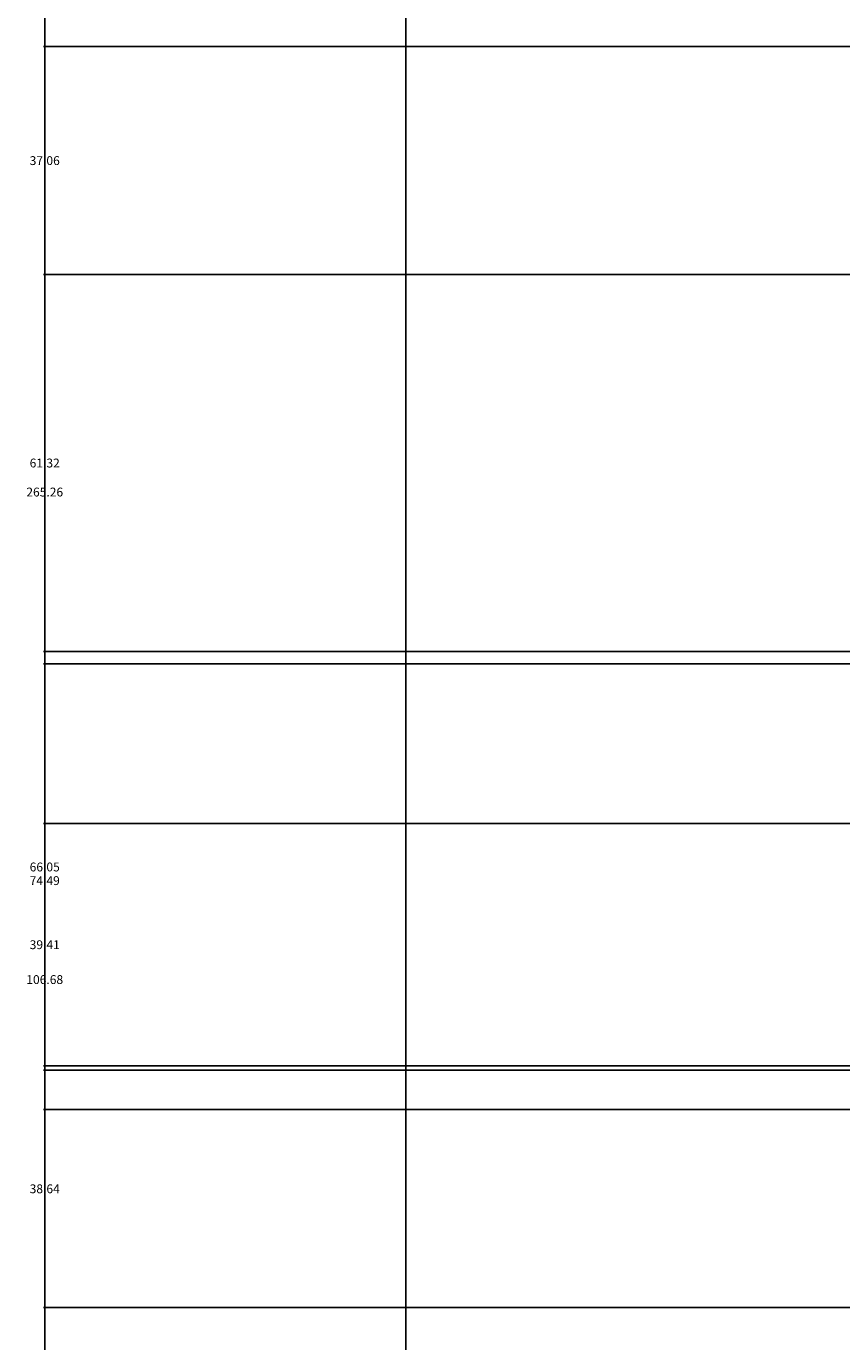
# Model space of a CAD drawing. Units: inches. Extents: x 241 to 943, y 109 to 1396.
# Tile 20 of 34: x 241 to 374, y 1065 to 1279. Entities that reach past the tile are written whole.
import ezdxf

# ---------------------------------------------------------------- set-up
doc = ezdxf.new("R2010")
doc.units = ezdxf.units.IN
doc.header["$MEASUREMENT"] = 0
doc.layers.add('A-ANNO-DIMS', color=2, linetype='Continuous', lineweight=18)
doc.styles.get("Standard").update_dxf_attribs({"font": 'arial.ttf'})
doc.dimstyles.get("Standard").update_dxf_attribs({"dimtxt": 1.4375, "dimasz": 0.18, "dimexe": 0.18, "dimexo": 0.0625, "dimgap": 0.09, "dimtad": 0, "dimtih": 1, "dimtoh": 1, "dimdec": 4, "dimzin": 0, "dimdsep": 46, "dimlunit": 4, "dimtxsty": 'Standard', "dimcen": 0.09, "dimadec": 0, "dimazin": 0, "dimtfac": 1, "dimtdec": 4, "dimtofl": 0, "dimtmove": 0, "dimatfit": 3, "dimfxl": 1, "dimtolj": 1, "dimtzin": 0, "dimarcsym": 0})

# ---------------------------------------------------------------- blocks, each defined once
blk = doc.blocks.new('*D5')
at = {"layer": 'A-ANNO-DIMS', "color": 0, "lineweight": -2, "transparency": 16777216}
for p, q in [((303.24, 177.8), (303.24, 1395.05)), ((303.42, 1394.87), (338.18, 1394.87)), ((376.86, 1394.87), (342.09, 1394.87)), ((377.04, 177.76), (377.04, 1395.05))]:
    blk.add_line(p, q, dxfattribs=at)
at = {"layer": 'A-ANNO-DIMS', "color": 0, "transparency": 16777216}
for points in [[(303.42, 1394.9), (303.42, 1394.84), (303.24, 1394.87)], [(376.86, 1394.9), (376.86, 1394.84), (377.04, 1394.87)]]:
    blk.add_solid(points, dxfattribs=at)
at = {"layer": 'Defpoints', "color": 0, "transparency": 16777216}
for p in [(377.04, 1394.87), (303.24, 177.74), (377.04, 177.7)]:
    blk.add_point(p, dxfattribs=at)
at = {"layer": 'A-ANNO-DIMS', "color": 0, "transparency": 16777216, "insert": (340.14, 1394.87), "char_height": 1.438, "attachment_point": 5}
blk.add_mtext('\\A1;73.8', dxfattribs=at)
blk = doc.blocks.new('*D7')
at = {"layer": 'A-ANNO-DIMS', "color": 0, "lineweight": -2, "transparency": 16777216}
for p, q in [((508.24, 1336.12), (244.31, 1336.12)), ((244.49, 1335.94), (244.49, 753.25)), ((244.49, 168.92), (244.49, 751.6)), ((303.17, 168.74), (244.31, 168.74))]:
    blk.add_line(p, q, dxfattribs=at)
at = {"layer": 'A-ANNO-DIMS', "color": 0, "transparency": 16777216}
for points in [[(244.46, 1335.94), (244.52, 1335.94), (244.49, 1336.12)], [(244.46, 168.92), (244.52, 168.92), (244.49, 168.74)]]:
    blk.add_solid(points, dxfattribs=at)
at = {"layer": 'Defpoints', "color": 0, "transparency": 16777216}
for p in [(244.49, 1336.12), (508.31, 1336.12), (303.24, 168.74)]:
    blk.add_point(p, dxfattribs=at)
at = {"layer": 'A-ANNO-DIMS', "color": 0, "transparency": 16777216, "insert": (244.49, 752.43), "char_height": 1.438, "attachment_point": 5}
blk.add_mtext('\\A1;1167.4', dxfattribs=at)
blk = doc.blocks.new('*D25')
at = {"layer": 'A-ANNO-DIMS', "color": 0, "lineweight": -2, "transparency": 16777216}
for p, q in [((376.98, 1070.85), (244.31, 1070.85)), ((244.49, 1070.67), (244.49, 1041.02)), ((244.49, 1009.72), (244.49, 1039.37)), ((376.98, 1009.54), (244.31, 1009.54))]:
    blk.add_line(p, q, dxfattribs=at)
at = {"layer": 'A-ANNO-DIMS', "color": 0, "transparency": 16777216}
for points in [[(244.46, 1070.67), (244.52, 1070.67), (244.49, 1070.85)], [(244.46, 1009.72), (244.52, 1009.72), (244.49, 1009.54)]]:
    blk.add_solid(points, dxfattribs=at)
at = {"layer": 'Defpoints', "color": 0, "transparency": 16777216}
for p in [(244.49, 1070.85), (377.04, 1070.85), (377.04, 1009.54)]:
    blk.add_point(p, dxfattribs=at)
at = {"layer": 'A-ANNO-DIMS', "color": 0, "transparency": 16777216, "insert": (244.49, 1040.2), "char_height": 1.438, "attachment_point": 5}
blk.add_mtext('\\A1;61.32', dxfattribs=at)
blk = doc.blocks.new('*D26')
at = {"layer": 'A-ANNO-DIMS', "color": 0, "lineweight": -2, "transparency": 16777216}
for p, q in [((376.98, 1177.54), (244.31, 1177.54)), ((244.49, 1177.36), (244.49, 1125.02)), ((244.49, 1071.03), (244.49, 1123.37)), ((376.98, 1070.85), (244.31, 1070.85))]:
    blk.add_line(p, q, dxfattribs=at)
at = {"layer": 'A-ANNO-DIMS', "color": 0, "transparency": 16777216}
for points in [[(244.46, 1177.36), (244.52, 1177.36), (244.49, 1177.54)], [(244.46, 1071.03), (244.52, 1071.03), (244.49, 1070.85)]]:
    blk.add_solid(points, dxfattribs=at)
at = {"layer": 'Defpoints', "color": 0, "transparency": 16777216}
for p in [(244.49, 1177.54), (377.04, 1177.54), (377.04, 1070.85)]:
    blk.add_point(p, dxfattribs=at)
at = {"layer": 'A-ANNO-DIMS', "color": 0, "transparency": 16777216, "insert": (244.49, 1124.2), "char_height": 1.438, "attachment_point": 5}
blk.add_mtext('\\A1;106.68', dxfattribs=at)
blk = doc.blocks.new('*D27')
at = {"layer": 'A-ANNO-DIMS', "color": 0, "lineweight": -2, "transparency": 16777216}
for p, q in [((376.98, 1238.85), (244.31, 1238.85)), ((244.49, 1238.67), (244.49, 1209.02)), ((244.49, 1177.72), (244.49, 1207.37)), ((376.98, 1177.54), (244.31, 1177.54))]:
    blk.add_line(p, q, dxfattribs=at)
at = {"layer": 'A-ANNO-DIMS', "color": 0, "transparency": 16777216}
for points in [[(244.46, 1238.67), (244.52, 1238.67), (244.49, 1238.85)], [(244.46, 1177.72), (244.52, 1177.72), (244.49, 1177.54)]]:
    blk.add_solid(points, dxfattribs=at)
at = {"layer": 'Defpoints', "color": 0, "transparency": 16777216}
for p in [(244.49, 1238.85), (377.04, 1238.85), (377.04, 1177.54)]:
    blk.add_point(p, dxfattribs=at)
at = {"layer": 'A-ANNO-DIMS', "color": 0, "transparency": 16777216, "insert": (244.49, 1208.2), "char_height": 1.438, "attachment_point": 5}
blk.add_mtext('\\A1;61.32', dxfattribs=at)
blk = doc.blocks.new('*D28')
at = {"layer": 'A-ANNO-DIMS', "color": 0, "lineweight": -2, "transparency": 16777216}
for p, q in [((376.98, 1275.91), (244.31, 1275.91)), ((244.49, 1275.73), (244.49, 1258.21)), ((244.49, 1239.03), (244.49, 1256.56)), ((376.98, 1238.85), (244.31, 1238.85))]:
    blk.add_line(p, q, dxfattribs=at)
at = {"layer": 'A-ANNO-DIMS', "color": 0, "transparency": 16777216}
for points in [[(244.46, 1275.73), (244.52, 1275.73), (244.49, 1275.91)], [(244.46, 1239.03), (244.52, 1239.03), (244.49, 1238.85)]]:
    blk.add_solid(points, dxfattribs=at)
at = {"layer": 'Defpoints', "color": 0, "transparency": 16777216}
for p in [(244.49, 1275.91), (377.04, 1275.91), (377.04, 1238.85)]:
    blk.add_point(p, dxfattribs=at)
at = {"layer": 'A-ANNO-DIMS', "color": 0, "transparency": 16777216, "insert": (244.49, 1257.38), "char_height": 1.438, "attachment_point": 5}
blk.add_mtext('\\A1;37.06', dxfattribs=at)
blk = doc.blocks.new('*D39')
at = {"layer": 'A-ANNO-DIMS', "color": 0, "lineweight": -2, "transparency": 16777216}
for p, q in [((388.98, 1109.49), (244.31, 1109.49)), ((244.49, 1109.31), (244.49, 1091)), ((244.49, 1071.03), (244.49, 1089.35)), ((388.98, 1070.85), (244.31, 1070.85))]:
    blk.add_line(p, q, dxfattribs=at)
at = {"layer": 'A-ANNO-DIMS', "color": 0, "transparency": 16777216}
for points in [[(244.46, 1109.31), (244.52, 1109.31), (244.49, 1109.49)], [(244.46, 1071.03), (244.52, 1071.03), (244.49, 1070.85)]]:
    blk.add_solid(points, dxfattribs=at)
at = {"layer": 'Defpoints', "color": 0, "transparency": 16777216}
for p in [(244.49, 1109.49), (389.04, 1109.49), (389.04, 1070.85)]:
    blk.add_point(p, dxfattribs=at)
at = {"layer": 'A-ANNO-DIMS', "color": 0, "transparency": 16777216, "insert": (244.49, 1090.17), "char_height": 1.438, "attachment_point": 5}
blk.add_mtext('\\A1;38.64', dxfattribs=at)
blk = doc.blocks.new('*D40')
at = {"layer": 'A-ANNO-DIMS', "color": 0, "lineweight": -2, "transparency": 16777216}
for p, q in [((398.25, 1175.54), (244.31, 1175.54)), ((244.49, 1175.36), (244.49, 1143.34)), ((244.49, 1109.67), (244.49, 1141.69)), ((396.25, 1109.49), (244.31, 1109.49))]:
    blk.add_line(p, q, dxfattribs=at)
at = {"layer": 'A-ANNO-DIMS', "color": 0, "transparency": 16777216}
for points in [[(244.46, 1175.36), (244.52, 1175.36), (244.49, 1175.54)], [(244.46, 1109.67), (244.52, 1109.67), (244.49, 1109.49)]]:
    blk.add_solid(points, dxfattribs=at)
at = {"layer": 'Defpoints', "color": 0, "transparency": 16777216}
for p in [(244.49, 1175.54), (398.31, 1175.54), (396.31, 1109.49)]:
    blk.add_point(p, dxfattribs=at)
at = {"layer": 'A-ANNO-DIMS', "color": 0, "transparency": 16777216, "insert": (244.49, 1142.51), "char_height": 1.438, "attachment_point": 5}
blk.add_mtext('\\A1;66.05', dxfattribs=at)
blk = doc.blocks.new('*D49')
at = {"layer": 'A-ANNO-DIMS', "color": 0, "lineweight": -2, "transparency": 16777216}
for p, q in [((766.24, 1177.54), (244.31, 1177.54)), ((244.49, 1177.36), (244.49, 1141.12)), ((244.49, 1103.23), (244.49, 1139.47)), ((766.24, 1103.05), (244.31, 1103.05))]:
    blk.add_line(p, q, dxfattribs=at)
at = {"layer": 'A-ANNO-DIMS', "color": 0, "transparency": 16777216}
for points in [[(244.46, 1177.36), (244.52, 1177.36), (244.49, 1177.54)], [(244.46, 1103.23), (244.52, 1103.23), (244.49, 1103.05)]]:
    blk.add_solid(points, dxfattribs=at)
at = {"layer": 'Defpoints', "color": 0, "transparency": 16777216}
for p in [(244.49, 1177.54), (766.3, 1177.54), (766.3, 1103.05)]:
    blk.add_point(p, dxfattribs=at)
at = {"layer": 'A-ANNO-DIMS', "color": 0, "transparency": 16777216, "insert": (244.49, 1140.29), "char_height": 1.438, "attachment_point": 5}
blk.add_mtext('\\A1;74.49', dxfattribs=at)
blk = doc.blocks.new('*D92')
at = {"layer": 'A-ANNO-DIMS', "color": 0, "lineweight": -2, "transparency": 16777216}
for p, q in [((508.24, 1336.12), (244.31, 1336.12)), ((244.49, 1335.94), (244.49, 1204.31)), ((244.49, 1071.03), (244.49, 1202.66)), ((508.24, 1070.85), (244.31, 1070.85))]:
    blk.add_line(p, q, dxfattribs=at)
at = {"layer": 'A-ANNO-DIMS', "color": 0, "transparency": 16777216}
for points in [[(244.46, 1335.94), (244.52, 1335.94), (244.49, 1336.12)], [(244.46, 1071.03), (244.52, 1071.03), (244.49, 1070.85)]]:
    blk.add_solid(points, dxfattribs=at)
at = {"layer": 'Defpoints', "color": 0, "transparency": 16777216}
for p in [(244.49, 1336.12), (508.31, 1336.12), (508.31, 1070.85)]:
    blk.add_point(p, dxfattribs=at)
at = {"layer": 'A-ANNO-DIMS', "color": 0, "transparency": 16777216, "insert": (244.49, 1203.48), "char_height": 1.438, "attachment_point": 5}
blk.add_mtext('\\A1;265.26', dxfattribs=at)
blk = doc.blocks.new('*D110')
at = {"layer": 'A-ANNO-DIMS', "color": 0, "lineweight": -2, "transparency": 16777216}
for p, q in [((535.89, 1149.58), (244.31, 1149.58)), ((244.49, 1149.4), (244.49, 1130.7)), ((244.49, 1110.35), (244.49, 1129.05)), ((535.89, 1110.17), (244.31, 1110.17))]:
    blk.add_line(p, q, dxfattribs=at)
at = {"layer": 'A-ANNO-DIMS', "color": 0, "transparency": 16777216}
for points in [[(244.46, 1149.4), (244.52, 1149.4), (244.49, 1149.58)], [(244.46, 1110.35), (244.52, 1110.35), (244.49, 1110.17)]]:
    blk.add_solid(points, dxfattribs=at)
at = {"layer": 'Defpoints', "color": 0, "transparency": 16777216}
for p in [(244.49, 1149.58), (535.95, 1149.58), (535.95, 1110.17)]:
    blk.add_point(p, dxfattribs=at)
at = {"layer": 'A-ANNO-DIMS', "color": 0, "transparency": 16777216, "insert": (244.49, 1129.87), "char_height": 1.438, "attachment_point": 5}
blk.add_mtext('\\A1;39.41', dxfattribs=at)

msp = doc.modelspace()

# ---------------------------------------------------------------- dimensions: what is measured, and where the dimension line sits
at = {"layer": 'A-ANNO-DIMS'}
dim = msp.add_linear_dim(base=(377.0391, 1394.8654), p1=(303.2358, 177.7407), p2=(377.0391, 177.6977), dimstyle='Standard', override={"dimdec": 1, "dimlfac": 1, "dimrnd": 0, "dimzin": 0, "dimdsep": 46, "dimlunit": 2}, dxfattribs=at)
dim.commit()
dim.dimension.update_dxf_attribs({"geometry": '*D5', "text_midpoint": (340.1375, 1394.8654)})
for base, p1, p2, override, picture, middle in [((244.4858, 1336.1154), (303.2358, 168.7407), (508.3064, 1336.1154), {"dimdec": 1, "dimlfac": 1, "dimrnd": 0, "dimzin": 0, "dimdsep": 46, "dimlunit": 2}, '*D7', (244.4858, 752.4281)), ((244.4858, 1336.1154), (508.3064, 1070.8538), (508.3064, 1336.1154), {"dimdec": 2, "dimlfac": 1, "dimrnd": 0, "dimzin": 0, "dimdsep": 46, "dimlunit": 2}, '*D92', (244.4858, 1203.4846)), ((244.4858, 1275.9142), (377.0391, 1238.8538), (377.0391, 1275.9142), {"dimdec": 2, "dimlfac": 1, "dimrnd": 0, "dimzin": 0, "dimdsep": 46, "dimlunit": 2}, '*D28', (244.4858, 1257.384)), ((244.4858, 1238.8538), (377.0391, 1177.5382), (377.0391, 1238.8538), {"dimdec": 2, "dimlfac": 1, "dimrnd": 0, "dimzin": 0, "dimdsep": 46, "dimlunit": 2}, '*D27', (244.4858, 1208.196)), ((244.4858, 1177.5382), (377.0391, 1070.8538), (377.0391, 1177.5382), {"dimdec": 2, "dimlfac": 1, "dimrnd": 0, "dimzin": 0, "dimdsep": 46, "dimlunit": 2}, '*D26', (244.4858, 1124.196)), ((244.4858, 1177.5382), (766.3038, 1103.0477), (766.3038, 1177.5382), {"dimdec": 2, "dimlfac": 1, "dimrnd": 0, "dimzin": 0, "dimdsep": 46, "dimlunit": 2}, '*D49', (244.4858, 1140.2929)), ((244.4858, 1175.5382), (396.3125, 1109.4916), (398.3125, 1175.5382), {"dimdec": 2, "dimlfac": 1, "dimrnd": 0, "dimzin": 0, "dimdsep": 46, "dimlunit": 2}, '*D40', (244.4858, 1142.5149)), ((244.4858, 1149.5772), (535.952, 1110.1686), (535.952, 1149.5772), {"dimdec": 2, "dimlfac": 1, "dimrnd": 0, "dimzin": 0, "dimdsep": 46, "dimlunit": 2}, '*D110', (244.4858, 1129.8729)), ((244.4858, 1109.4916), (389.0429, 1070.8538), (389.0429, 1109.4916), {"dimdec": 2, "dimlfac": 1, "dimrnd": 0, "dimzin": 0, "dimdsep": 46, "dimlunit": 2}, '*D39', (244.4858, 1090.1727)), ((244.4858, 1070.8538), (377.0391, 1009.5382), (377.0391, 1070.8538), {"dimdec": 2, "dimlfac": 1, "dimrnd": 0, "dimzin": 0, "dimdsep": 46, "dimlunit": 2}, '*D25', (244.4858, 1040.196))]:
    dim = msp.add_linear_dim(base=base, p1=p1, p2=p2, angle=90, dimstyle='Standard', override=override, dxfattribs=at)
    dim.commit()
    dim.dimension.update_dxf_attribs({"geometry": picture, "text_midpoint": middle})

doc.saveas('drawing.dxf')
